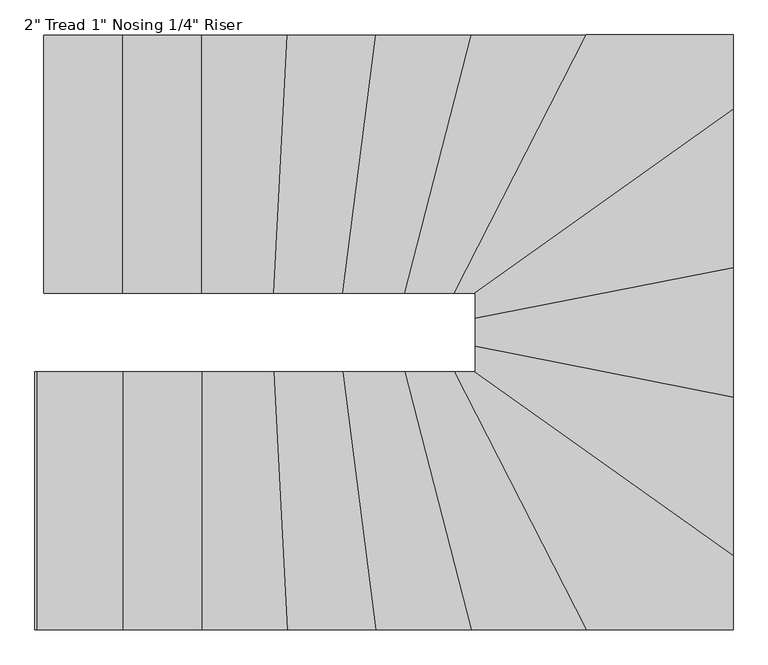
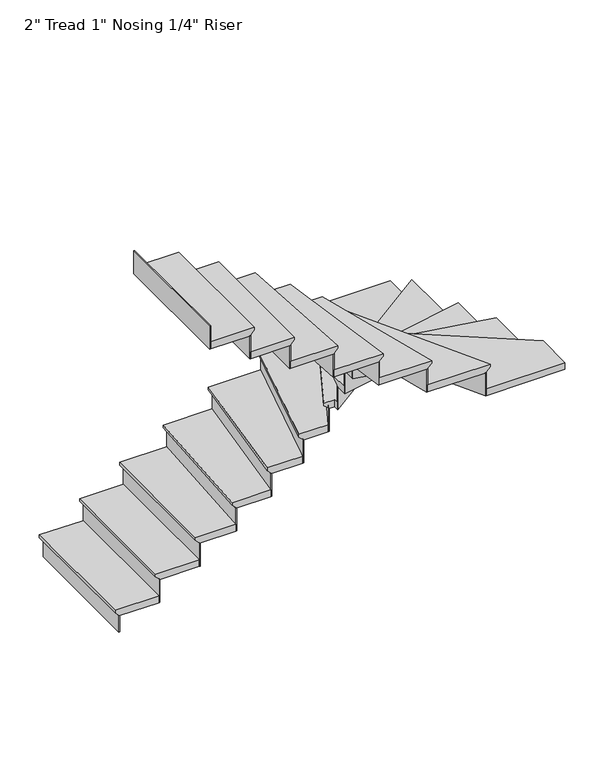
"""IFC4 building model written with IfcOpenShell, lengths in millimetres: stair flight geometry."""

from ifc_helpers import new_model, si_unit, origin, place, context, project, spatial, faceted_brep, source, transform, mapped, element, save


def stair_flight_f23435a1(model_context):
    return source(origin(), model_context, "Body", "Brep", [
        faceted_brep([(306.9570026, -4376.7064015, 150.2833333), (306.9570026, -4376.7064015, 169.3333333), (306.9570026, -3462.3064015, 169.3333333), (306.9570026, -3462.3064015, 150.2833333), (332.3570026, -4376.7064015, 124.8833333), (332.3570026, -3462.3064015, 124.8833333), (611.7570026, -4376.7064015, 169.3333333), (611.7570026, -3462.3064015, 169.3333333), (332.3570026, -3462.3064015, 118.5333333), (611.7570026, -3462.3064015, 118.5333333), (611.7570026, -4376.7064015, 118.5333333), (332.3570026, -4376.7064015, 118.5333333)], [[[0, 1, 2, 3]], [[4, 0, 3, 5]], [[2, 1, 6, 7]], [[8, 9, 10, 11]], [[2, 7, 9, 8, 5, 3]], [[8, 11, 4, 5]], [[6, 1, 0, 4, 11, 10]], [[7, 6, 10, 9]]]),
        faceted_brep([(332.3570026, -4376.7064015, 118.5333333), (332.3570026, -4376.7064015, 0.0), (338.7070026, -4376.7064015, 0.0), (338.7070026, -4376.7064015, 118.5333333), (332.3570026, -3462.3064015, 118.5333333), (338.7070026, -3462.3064015, 118.5333333), (338.7070026, -3462.3064015, 0.0), (332.3570026, -3462.3064015, 0.0)], [[[0, 1, 2, 3]], [[4, 5, 6, 7]], [[1, 0, 4, 7]], [[2, 1, 7, 6]], [[3, 2, 6, 5]], [[0, 3, 5, 4]]]),
        faceted_brep([(611.7570026, -4376.7064015, 287.8666667), (611.7570026, -4376.7064015, 118.5333333), (618.1070026, -4376.7064015, 118.5333333), (618.1070026, -4376.7064015, 287.8666667), (611.7570026, -3462.3064015, 287.8666667), (618.1070026, -3462.3064015, 287.8666667), (618.1070026, -3462.3064015, 118.5333333), (611.7570026, -3462.3064015, 118.5333333)], [[[0, 1, 2, 3]], [[4, 5, 6, 7]], [[1, 0, 4, 7]], [[2, 1, 7, 6]], [[3, 2, 6, 5]], [[0, 3, 5, 4]]]),
        faceted_brep([(586.3570026, -3462.3064015, 338.6666667), (586.3570026, -4376.7064015, 338.6666667), (891.1570026, -4376.7064015, 338.6666667), (891.1570026, -3462.3064015, 338.6666667), (611.7570026, -3462.3064015, 287.8666667), (891.1570026, -3462.3064015, 287.8666667), (891.1570026, -4376.7064015, 287.8666667), (611.7570026, -4376.7064015, 287.8666667), (611.7570026, -3462.3064015, 294.2166667), (586.3570026, -3462.3064015, 319.6166667), (611.7570026, -4376.7064015, 294.2166667), (586.3570026, -4376.7064015, 319.6166667)], [[[0, 1, 2, 3]], [[4, 5, 6, 7]], [[0, 3, 5, 4, 8, 9]], [[4, 7, 10, 8]], [[2, 1, 11, 10, 7, 6]], [[3, 2, 6, 5]], [[11, 1, 0, 9]], [[10, 11, 9, 8]]]),
        faceted_brep([(891.1570026, -4376.7064015, 457.2), (891.1570026, -4376.7064015, 287.8666667), (897.5070026, -4376.7064015, 287.8666667), (897.5070026, -4376.7064015, 457.2), (891.1570026, -3462.3064015, 457.2), (897.5070026, -3462.3064015, 457.2), (897.5070026, -3462.3064015, 287.8666667), (891.1570026, -3462.3064015, 287.8666667)], [[[0, 1, 2, 3]], [[4, 5, 6, 7]], [[1, 0, 4, 7]], [[2, 1, 7, 6]], [[3, 2, 6, 5]], [[0, 3, 5, 4]]]),
        faceted_brep([(865.7570026, -3462.3064015, 508.0), (865.7570026, -4376.7064015, 508.0), (1146.824164, -4376.7064015, 508.0), (1194.3584344, -3462.3064015, 508.0), (891.1570026, -3462.3064015, 457.2), (1194.3584344, -3462.3064015, 457.2), (1146.824164, -4376.7064015, 457.2), (891.1570026, -4376.7064015, 457.2), (891.1570026, -3462.3064015, 463.55), (865.7570026, -3462.3064015, 488.95), (891.1570026, -4376.7064015, 463.55), (865.7570026, -4376.7064015, 488.95)], [[[0, 1, 2, 3]], [[4, 5, 6, 7]], [[0, 3, 5, 4, 8, 9]], [[4, 7, 10, 8]], [[2, 1, 11, 10, 7, 6]], [[3, 2, 6, 5]], [[11, 1, 0, 9]], [[10, 11, 9, 8]]]),
        faceted_brep([(1146.824164, -4376.7064015, 626.5333333), (1146.824164, -4376.7064015, 457.2), (1153.1827382, -4376.7064015, 457.2), (1153.1827382, -4376.7064015, 626.5333333), (1194.3584344, -3462.3064015, 626.5333333), (1200.7170086, -3462.3064015, 626.5333333), (1200.7170086, -3462.3064015, 457.2), (1194.3584344, -3462.3064015, 457.2)], [[[0, 1, 2, 3]], [[4, 5, 6, 7]], [[1, 0, 4, 7]], [[2, 1, 7, 6]], [[3, 2, 6, 5]], [[0, 3, 5, 4]]]),
        faceted_brep([(1168.9241378, -3462.3064015, 677.3333333), (1121.3898673, -4376.7064015, 677.3333333), (1390.9908638, -4376.7064015, 677.3333333), (1509.3469155, -3462.3064015, 677.3333333), (1194.3584344, -3462.3064015, 626.5333333), (1509.3469155, -3462.3064015, 626.5333333), (1390.9908638, -4376.7064015, 626.5333333), (1146.824164, -4376.7064015, 626.5333333), (1194.3584344, -3462.3064015, 632.8833333), (1168.9241378, -3462.3064015, 658.2833333), (1146.824164, -4376.7064015, 632.8833333), (1121.3898673, -4376.7064015, 658.2833333)], [[[0, 1, 2, 3]], [[4, 5, 6, 7]], [[0, 3, 5, 4, 8, 9]], [[4, 7, 10, 8]], [[2, 1, 11, 10, 7, 6]], [[3, 2, 6, 5]], [[11, 1, 0, 9]], [[10, 11, 9, 8]]]),
        faceted_brep([(1390.9908638, -4376.7064015, 795.8666667), (1390.9908638, -4376.7064015, 626.5333333), (1397.3938356, -4376.7064015, 626.5333333), (1397.3938356, -4376.7064015, 795.8666667), (1509.3469155, -3462.3064015, 795.8666667), (1515.7498873, -3462.3064015, 795.8666667), (1515.7498873, -3462.3064015, 626.5333333), (1509.3469155, -3462.3064015, 626.5333333)], [[[0, 1, 2, 3]], [[4, 5, 6, 7]], [[1, 0, 4, 7]], [[2, 1, 7, 6]], [[3, 2, 6, 5]], [[0, 3, 5, 4]]]),
        faceted_brep([(1483.7350284, -3462.3064015, 846.6666667), (1365.3789767, -4376.7064015, 846.6666667), (1612.6180863, -4376.7064015, 846.6666667), (1847.7485337, -3462.3064015, 846.6666667), (1509.3469155, -3462.3064015, 795.8666667), (1847.7485337, -3462.3064015, 795.8666667), (1612.6180863, -4376.7064015, 795.8666667), (1390.9908638, -4376.7064015, 795.8666667), (1509.3469155, -3462.3064015, 802.2166667), (1483.7350284, -3462.3064015, 827.6166667), (1390.9908638, -4376.7064015, 802.2166667), (1365.3789767, -4376.7064015, 827.6166667)], [[[0, 1, 2, 3]], [[4, 5, 6, 7]], [[0, 3, 5, 4, 8, 9]], [[4, 7, 10, 8]], [[2, 1, 11, 10, 7, 6]], [[3, 2, 6, 5]], [[11, 1, 0, 9]], [[10, 11, 9, 8]]]),
        faceted_brep([(1612.6180863, -4376.7064015, 965.2), (1612.6180863, -4376.7064015, 795.8666667), (1619.1746632, -4376.7064015, 795.8666667), (1619.1746632, -4376.7064015, 965.2), (1847.7485337, -3462.3064015, 965.2), (1854.3051106, -3462.3064015, 965.2), (1854.3051106, -3462.3064015, 795.8666667), (1847.7485337, -3462.3064015, 795.8666667)], [[[0, 1, 2, 3]], [[4, 5, 6, 7]], [[1, 0, 4, 7]], [[2, 1, 7, 6]], [[3, 2, 6, 5]], [[0, 3, 5, 4]]]),
        faceted_brep([(1821.5222263, -3462.3064015, 1016.0), (1586.3917788, -4376.7064015, 1016.0), (1788.9647224, -4376.7064015, 1016.0), (2257.7893437, -3462.3064015, 1016.0), (1847.7485337, -3462.3064015, 965.2), (2257.7893437, -3462.3064015, 965.2), (1788.9647224, -4376.7064015, 965.2), (1612.6180863, -4376.7064015, 965.2), (1847.7485337, -3462.3064015, 971.55), (1821.5222263, -3462.3064015, 996.95), (1612.6180863, -4376.7064015, 971.55), (1586.3917788, -4376.7064015, 996.95)], [[[0, 1, 2, 3]], [[4, 5, 6, 7]], [[0, 3, 5, 4, 8, 9]], [[4, 7, 10, 8]], [[2, 1, 11, 10, 7, 6]], [[3, 2, 6, 5]], [[11, 1, 0, 9]], [[10, 11, 9, 8]]]),
        faceted_brep([(1788.9647224, -4376.7064015, 1134.5333333), (1788.9647224, -4376.7064015, 965.2), (1796.1007055, -4376.7064015, 965.2), (1796.1007055, -4376.7064015, 1134.5333333), (2257.7893437, -3462.3064015, 1134.5333333), (2264.9253269, -3462.3064015, 1134.5333333), (2264.9253269, -3462.3064015, 965.2), (2257.7893437, -3462.3064015, 965.2)], [[[0, 1, 2, 3]], [[4, 5, 6, 7]], [[1, 0, 4, 7]], [[2, 1, 7, 6]], [[3, 2, 6, 5]], [[0, 3, 5, 4]]]),
        faceted_brep([(2749.0886944, -3755.9875352, 1185.3333333), (2749.0886944, -3462.3064015, 1185.3333333), (2229.2454112, -3462.3064015, 1185.3333333), (1760.4207899, -4376.7064015, 1185.3333333), (1834.6886944, -4376.7064015, 1185.3333333), (1834.6886944, -4406.2614844, 1185.3333333), (2749.0886944, -3462.3064015, 1134.5333333), (2749.0886944, -3755.9875352, 1134.5333333), (1834.6886944, -4406.2614844, 1134.5333333), (1834.6886944, -4376.7064015, 1134.5333333), (1788.9647224, -4376.7064015, 1134.5333333), (2257.7893437, -3462.3064015, 1134.5333333), (2257.7893437, -3462.3064015, 1140.8833333), (2229.2454112, -3462.3064015, 1166.2833333), (1788.9647224, -4376.7064015, 1140.8833333), (1760.4207899, -4376.7064015, 1166.2833333)], [[[0, 1, 2, 3, 4, 5]], [[6, 7, 8, 9, 10, 11]], [[1, 0, 7, 6]], [[2, 1, 6, 11, 12, 13]], [[11, 10, 14, 12]], [[4, 3, 15, 14, 10, 9]], [[5, 4, 9, 8]], [[0, 5, 8, 7]], [[15, 3, 2, 13]], [[14, 15, 13, 12]]]),
        faceted_brep([(1834.6886944, -4406.2614844, 1303.8666667), (1834.6886944, -4406.2614844, 1134.5333333), (1834.6886944, -4414.0534592, 1134.5333333), (1834.6886944, -4414.0534592, 1303.8666667), (2749.0886944, -3755.9875352, 1303.8666667), (2749.0886944, -3763.77951, 1303.8666667), (2749.0886944, -3763.77951, 1134.5333333), (2749.0886944, -3755.9875352, 1134.5333333)], [[[0, 1, 2, 3]], [[4, 5, 6, 7]], [[1, 0, 4, 7]], [[2, 1, 7, 6]], [[3, 2, 6, 5]], [[0, 3, 5, 4]]]),
        faceted_brep([(2749.0886944, -3724.819636, 1354.6666667), (1834.6886944, -4375.0935852, 1354.6666667), (1834.6886944, -4492.7155714, 1354.6666667), (2749.0886944, -4312.4747151, 1354.6666667), (2749.0886944, -3755.9875352, 1303.8666667), (2749.0886944, -4312.4747151, 1303.8666667), (1834.6886944, -4492.7155714, 1303.8666667), (1834.6886944, -4406.2614844, 1303.8666667), (2749.0886944, -3755.9875352, 1310.2166667), (2749.0886944, -3724.819636, 1335.6166667), (1834.6886944, -4406.2614844, 1310.2166667), (1834.6886944, -4375.0935852, 1335.6166667)], [[[0, 1, 2, 3]], [[4, 5, 6, 7]], [[0, 3, 5, 4, 8, 9]], [[4, 7, 10, 8]], [[2, 1, 11, 10, 7, 6]], [[3, 2, 6, 5]], [[11, 1, 0, 9]], [[10, 11, 9, 8]]]),
        faceted_brep([(1834.6886944, -4492.7155714, 1473.2), (1834.6886944, -4492.7155714, 1303.8666667), (1834.6886944, -4499.1877569, 1303.8666667), (1834.6886944, -4499.1877569, 1473.2), (2749.0886944, -4312.4747151, 1473.2), (2749.0886944, -4318.9469005, 1473.2), (2749.0886944, -4318.9469005, 1303.8666667), (2749.0886944, -4312.4747151, 1303.8666667)], [[[0, 1, 2, 3]], [[4, 5, 6, 7]], [[1, 0, 4, 7]], [[2, 1, 7, 6]], [[3, 2, 6, 5]], [[0, 3, 5, 4]]]),
        faceted_brep([(2749.0886944, -4286.5859733, 1524.0), (1834.6886944, -4466.8268297, 1524.0), (1834.6886944, -4591.8747151, 1524.0), (2749.0886944, -4772.1155714, 1524.0), (2749.0886944, -4312.4747151, 1473.2), (2749.0886944, -4772.1155714, 1473.2), (1834.6886944, -4591.8747151, 1473.2), (1834.6886944, -4492.7155714, 1473.2), (2749.0886944, -4312.4747151, 1479.55), (2749.0886944, -4286.5859733, 1504.95), (1834.6886944, -4492.7155714, 1479.55), (1834.6886944, -4466.8268297, 1504.95)], [[[0, 1, 2, 3]], [[4, 5, 6, 7]], [[0, 3, 5, 4, 8, 9]], [[4, 7, 10, 8]], [[2, 1, 11, 10, 7, 6]], [[3, 2, 6, 5]], [[11, 1, 0, 9]], [[10, 11, 9, 8]]]),
        faceted_brep([(1834.6886944, -4591.8747151, 1642.5333333), (1834.6886944, -4591.8747151, 1473.2), (1834.6886944, -4598.3469005, 1473.2), (1834.6886944, -4598.3469005, 1642.5333333), (2749.0886944, -4772.1155714, 1642.5333333), (2749.0886944, -4778.5877569, 1642.5333333), (2749.0886944, -4778.5877569, 1473.2), (2749.0886944, -4772.1155714, 1473.2)], [[[0, 1, 2, 3]], [[4, 5, 6, 7]], [[1, 0, 4, 7]], [[2, 1, 7, 6]], [[3, 2, 6, 5]], [[0, 3, 5, 4]]]),
        faceted_brep([(2749.0886944, -4746.2268297, 1693.3333333), (1834.6886944, -4565.9859733, 1693.3333333), (1834.6886944, -4656.1064015, 1693.3333333), (1788.5932199, -4656.1064015, 1693.3333333), (2749.0886944, -5339.1610662, 1693.3333333), (2749.0886944, -4772.1155714, 1642.5333333), (2749.0886944, -5339.1610662, 1642.5333333), (1788.5932199, -4656.1064015, 1642.5333333), (1834.6886944, -4656.1064015, 1642.5333333), (1834.6886944, -4591.8747151, 1642.5333333), (2749.0886944, -4772.1155714, 1648.8833333), (2749.0886944, -4746.2268297, 1674.2833333), (1834.6886944, -4591.8747151, 1648.8833333), (1834.6886944, -4565.9859733, 1674.2833333)], [[[0, 1, 2, 3, 4]], [[5, 6, 7, 8, 9]], [[0, 4, 6, 5, 10, 11]], [[5, 9, 12, 10]], [[2, 1, 13, 12, 9, 8]], [[3, 2, 8, 7]], [[4, 3, 7, 6]], [[13, 1, 0, 11]], [[12, 13, 11, 10]]]),
        faceted_brep([(1788.5932199, -4656.1064015, 1811.8666667), (1788.5932199, -4656.1064015, 1642.5333333), (1777.6363274, -4656.1064015, 1642.5333333), (1777.6363274, -4656.1064015, 1811.8666667), (2749.0886944, -5339.1610662, 1811.8666667), (2749.0886944, -5346.953041, 1811.8666667), (2749.0886944, -5346.953041, 1642.5333333), (2749.0886944, -5339.1610662, 1642.5333333)], [[[0, 1, 2, 3]], [[4, 5, 6, 7]], [[1, 0, 4, 7]], [[2, 1, 7, 6]], [[3, 2, 6, 5]], [[0, 3, 5, 4]]]),
        faceted_brep([(2200.7014787, -5570.5064015, 1862.6666667), (2749.0886944, -5570.5064015, 1862.6666667), (2749.0886944, -5307.993167, 1862.6666667), (1832.4207899, -4656.1064015, 1862.6666667), (1731.8768573, -4656.1064015, 1862.6666667), (2749.0886944, -5570.5064015, 1811.8666667), (2200.7014787, -5570.5064015, 1811.8666667), (1731.8768573, -4656.1064015, 1811.8666667), (1788.5932199, -4656.1064015, 1811.8666667), (2749.0886944, -5339.1610662, 1811.8666667), (2749.0886944, -5339.1610662, 1818.2166667), (2749.0886944, -5307.993167, 1843.6166667), (1788.5932199, -4656.1064015, 1818.2166667), (1832.4207899, -4656.1064015, 1843.6166667)], [[[0, 1, 2, 3, 4]], [[5, 6, 7, 8, 9]], [[1, 0, 6, 5]], [[2, 1, 5, 9, 10, 11]], [[9, 8, 12, 10]], [[4, 3, 13, 12, 8, 7]], [[0, 4, 7, 6]], [[13, 3, 2, 11]], [[12, 13, 11, 10]]]),
        faceted_brep([(1731.8768573, -4656.1064015, 1981.2), (1731.8768573, -4656.1064015, 1811.8666667), (1724.7408742, -4656.1064015, 1811.8666667), (1724.7408742, -4656.1064015, 1981.2), (2200.7014787, -5570.5064015, 1981.2), (2193.5654955, -5570.5064015, 1981.2), (2193.5654955, -5570.5064015, 1811.8666667), (2200.7014787, -5570.5064015, 1811.8666667)], [[[0, 1, 2, 3]], [[4, 5, 6, 7]], [[1, 0, 4, 7]], [[2, 1, 7, 6]], [[3, 2, 6, 5]], [[0, 3, 5, 4]]]),
        faceted_brep([(2229.2454112, -5570.5064015, 2032.0), (1760.4207899, -4656.1064015, 2032.0), (1560.1654714, -4656.1064015, 2032.0), (1795.2959188, -5570.5064015, 2032.0), (2200.7014787, -5570.5064015, 1981.2), (1795.2959188, -5570.5064015, 1981.2), (1560.1654714, -4656.1064015, 1981.2), (1731.8768573, -4656.1064015, 1981.2), (2200.7014787, -5570.5064015, 1987.55), (2229.2454112, -5570.5064015, 2012.95), (1731.8768573, -4656.1064015, 1987.55), (1760.4207899, -4656.1064015, 2012.95)], [[[0, 1, 2, 3]], [[4, 5, 6, 7]], [[0, 3, 5, 4, 8, 9]], [[4, 7, 10, 8]], [[2, 1, 11, 10, 7, 6]], [[3, 2, 6, 5]], [[11, 1, 0, 9]], [[10, 11, 9, 8]]]),
        faceted_brep([(1560.1654714, -4656.1064015, 2150.5333333), (1560.1654714, -4656.1064015, 1981.2), (1553.6088945, -4656.1064015, 1981.2), (1553.6088945, -4656.1064015, 2150.5333333), (1795.2959188, -5570.5064015, 2150.5333333), (1788.7393419, -5570.5064015, 2150.5333333), (1788.7393419, -5570.5064015, 1981.2), (1795.2959188, -5570.5064015, 1981.2)], [[[0, 1, 2, 3]], [[4, 5, 6, 7]], [[1, 0, 4, 7]], [[2, 1, 7, 6]], [[3, 2, 6, 5]], [[0, 3, 5, 4]]]),
        faceted_brep([(1821.5222263, -5570.5064015, 2201.3333333), (1586.3917788, -4656.1064015, 2201.3333333), (1339.7670896, -4656.1064015, 2201.3333333), (1458.1231413, -5570.5064015, 2201.3333333), (1795.2959188, -5570.5064015, 2150.5333333), (1458.1231413, -5570.5064015, 2150.5333333), (1339.7670896, -4656.1064015, 2150.5333333), (1560.1654714, -4656.1064015, 2150.5333333), (1795.2959188, -5570.5064015, 2156.8833333), (1821.5222263, -5570.5064015, 2182.2833333), (1560.1654714, -4656.1064015, 2156.8833333), (1586.3917788, -4656.1064015, 2182.2833333)], [[[0, 1, 2, 3]], [[4, 5, 6, 7]], [[0, 3, 5, 4, 8, 9]], [[4, 7, 10, 8]], [[2, 1, 11, 10, 7, 6]], [[3, 2, 6, 5]], [[11, 1, 0, 9]], [[10, 11, 9, 8]]]),
        faceted_brep([(1339.7670896, -4656.1064015, 2319.8666667), (1339.7670896, -4656.1064015, 2150.5333333), (1333.3641178, -4656.1064015, 2150.5333333), (1333.3641178, -4656.1064015, 2319.8666667), (1458.1231413, -5570.5064015, 2319.8666667), (1451.7201695, -5570.5064015, 2319.8666667), (1451.7201695, -5570.5064015, 2150.5333333), (1458.1231413, -5570.5064015, 2150.5333333)], [[[0, 1, 2, 3]], [[4, 5, 6, 7]], [[1, 0, 4, 7]], [[2, 1, 7, 6]], [[3, 2, 6, 5]], [[0, 3, 5, 4]]]),
        faceted_brep([(1483.7350284, -5570.5064015, 2370.6666667), (1365.3789767, -4656.1064015, 2370.6666667), (1095.9555707, -4656.1064015, 2370.6666667), (1143.4898411, -5570.5064015, 2370.6666667), (1458.1231413, -5570.5064015, 2319.8666667), (1143.4898411, -5570.5064015, 2319.8666667), (1095.9555707, -4656.1064015, 2319.8666667), (1339.7670896, -4656.1064015, 2319.8666667), (1458.1231413, -5570.5064015, 2326.2166667), (1483.7350284, -5570.5064015, 2351.6166667), (1339.7670896, -4656.1064015, 2326.2166667), (1365.3789767, -4656.1064015, 2351.6166667)], [[[0, 1, 2, 3]], [[4, 5, 6, 7]], [[0, 3, 5, 4, 8, 9]], [[4, 7, 10, 8]], [[2, 1, 11, 10, 7, 6]], [[3, 2, 6, 5]], [[11, 1, 0, 9]], [[10, 11, 9, 8]]]),
        faceted_brep([(1095.9555707, -4656.1064015, 2489.2), (1095.9555707, -4656.1064015, 2319.8666667), (1089.5969965, -4656.1064015, 2319.8666667), (1089.5969965, -4656.1064015, 2489.2), (1143.4898411, -5570.5064015, 2489.2), (1137.1312669, -5570.5064015, 2489.2), (1137.1312669, -5570.5064015, 2319.8666667), (1143.4898411, -5570.5064015, 2319.8666667)], [[[0, 1, 2, 3]], [[4, 5, 6, 7]], [[1, 0, 4, 7]], [[2, 1, 7, 6]], [[3, 2, 6, 5]], [[0, 3, 5, 4]]]),
        faceted_brep([(1168.9241378, -5570.5064015, 2540.0), (1121.3898673, -4656.1064015, 2540.0), (840.3570026, -4656.1064015, 2540.0), (840.3570026, -5570.5064015, 2540.0), (1143.4898411, -5570.5064015, 2489.2), (840.3570026, -5570.5064015, 2489.2), (840.3570026, -4656.1064015, 2489.2), (1095.9555707, -4656.1064015, 2489.2), (1143.4898411, -5570.5064015, 2495.55), (1168.9241378, -5570.5064015, 2520.95), (1095.9555707, -4656.1064015, 2495.55), (1121.3898673, -4656.1064015, 2520.95)], [[[0, 1, 2, 3]], [[4, 5, 6, 7]], [[0, 3, 5, 4, 8, 9]], [[4, 7, 10, 8]], [[2, 1, 11, 10, 7, 6]], [[3, 2, 6, 5]], [[11, 1, 0, 9]], [[10, 11, 9, 8]]]),
        faceted_brep([(840.3570026, -4656.1064015, 2658.5333333), (840.3570026, -4656.1064015, 2489.2), (834.0070026, -4656.1064015, 2489.2), (834.0070026, -4656.1064015, 2658.5333333), (840.3570026, -5570.5064015, 2658.5333333), (834.0070026, -5570.5064015, 2658.5333333), (834.0070026, -5570.5064015, 2489.2), (840.3570026, -5570.5064015, 2489.2)], [[[0, 1, 2, 3]], [[4, 5, 6, 7]], [[1, 0, 4, 7]], [[2, 1, 7, 6]], [[3, 2, 6, 5]], [[0, 3, 5, 4]]]),
        faceted_brep([(865.7570026, -5570.5064015, 2709.3333333), (865.7570026, -4656.1064015, 2709.3333333), (560.9570026, -4656.1064015, 2709.3333333), (560.9570026, -5570.5064015, 2709.3333333), (840.3570026, -5570.5064015, 2658.5333333), (560.9570026, -5570.5064015, 2658.5333333), (560.9570026, -4656.1064015, 2658.5333333), (840.3570026, -4656.1064015, 2658.5333333), (840.3570026, -5570.5064015, 2664.8833333), (865.7570026, -5570.5064015, 2690.2833333), (840.3570026, -4656.1064015, 2664.8833333), (865.7570026, -4656.1064015, 2690.2833333)], [[[0, 1, 2, 3]], [[4, 5, 6, 7]], [[0, 3, 5, 4, 8, 9]], [[4, 7, 10, 8]], [[2, 1, 11, 10, 7, 6]], [[3, 2, 6, 5]], [[11, 1, 0, 9]], [[10, 11, 9, 8]]]),
        faceted_brep([(560.9570026, -4656.1064015, 2827.8666667), (560.9570026, -4656.1064015, 2658.5333333), (554.6070026, -4656.1064015, 2658.5333333), (554.6070026, -4656.1064015, 2827.8666667), (560.9570026, -5570.5064015, 2827.8666667), (554.6070026, -5570.5064015, 2827.8666667), (554.6070026, -5570.5064015, 2658.5333333), (560.9570026, -5570.5064015, 2658.5333333)], [[[0, 1, 2, 3]], [[4, 5, 6, 7]], [[1, 0, 4, 7]], [[2, 1, 7, 6]], [[3, 2, 6, 5]], [[0, 3, 5, 4]]]),
        faceted_brep([(281.5570026, -4656.1064015, 2997.2), (281.5570026, -4656.1064015, 2827.8666667), (275.2070026, -4656.1064015, 2827.8666667), (275.2070026, -4656.1064015, 2997.2), (281.5570026, -5570.5064015, 2997.2), (275.2070026, -5570.5064015, 2997.2), (275.2070026, -5570.5064015, 2827.8666667), (281.5570026, -5570.5064015, 2827.8666667)], [[[0, 1, 2, 3]], [[4, 5, 6, 7]], [[1, 0, 4, 7]], [[2, 1, 7, 6]], [[3, 2, 6, 5]], [[0, 3, 5, 4]]]),
        faceted_brep([(586.3570026, -5570.5064015, 2878.6666667), (586.3570026, -4656.1064015, 2878.6666667), (281.5570026, -4656.1064015, 2878.6666667), (281.5570026, -5570.5064015, 2878.6666667), (560.9570026, -5570.5064015, 2827.8666667), (281.5570026, -5570.5064015, 2827.8666667), (281.5570026, -4656.1064015, 2827.8666667), (560.9570026, -4656.1064015, 2827.8666667), (560.9570026, -5570.5064015, 2834.2166667), (586.3570026, -5570.5064015, 2859.6166667), (560.9570026, -4656.1064015, 2834.2166667), (586.3570026, -4656.1064015, 2859.6166667)], [[[0, 1, 2, 3]], [[4, 5, 6, 7]], [[0, 3, 5, 4, 8, 9]], [[4, 7, 10, 8]], [[2, 1, 11, 10, 7, 6]], [[3, 2, 6, 5]], [[11, 1, 0, 9]], [[10, 11, 9, 8]]]),
    ])


if __name__ == "__main__":
    model = new_model("IFC4")
    model_context = context("Model", 3, world=origin())
    ifc_project = project(units=[si_unit("LENGTHUNIT", "METRE", prefix="MILLI")], contexts=[model_context])
    site = spatial("IfcSite", under=ifc_project)
    building = spatial("IfcBuilding", under=site)
    placement = place(None, origin())
    stair_flight_shape = stair_flight_f23435a1(model_context)
    element("IfcStairFlight", 1, ObjectType="2\" Tread 1\" Nosing 1/4\" Riser", at=placement, inside=building, context=model_context, shape_type="MappedRepresentation", body=[
        mapped(stair_flight_shape, transform((0.0, 0.0, 0.0), x_axis=(1.0, 0.0, 0.0), y_axis=(0.0, 1.0, 0.0), z_axis=(0.0, 0.0, 1.0))),
    ])
    save(model, "model.ifc")
